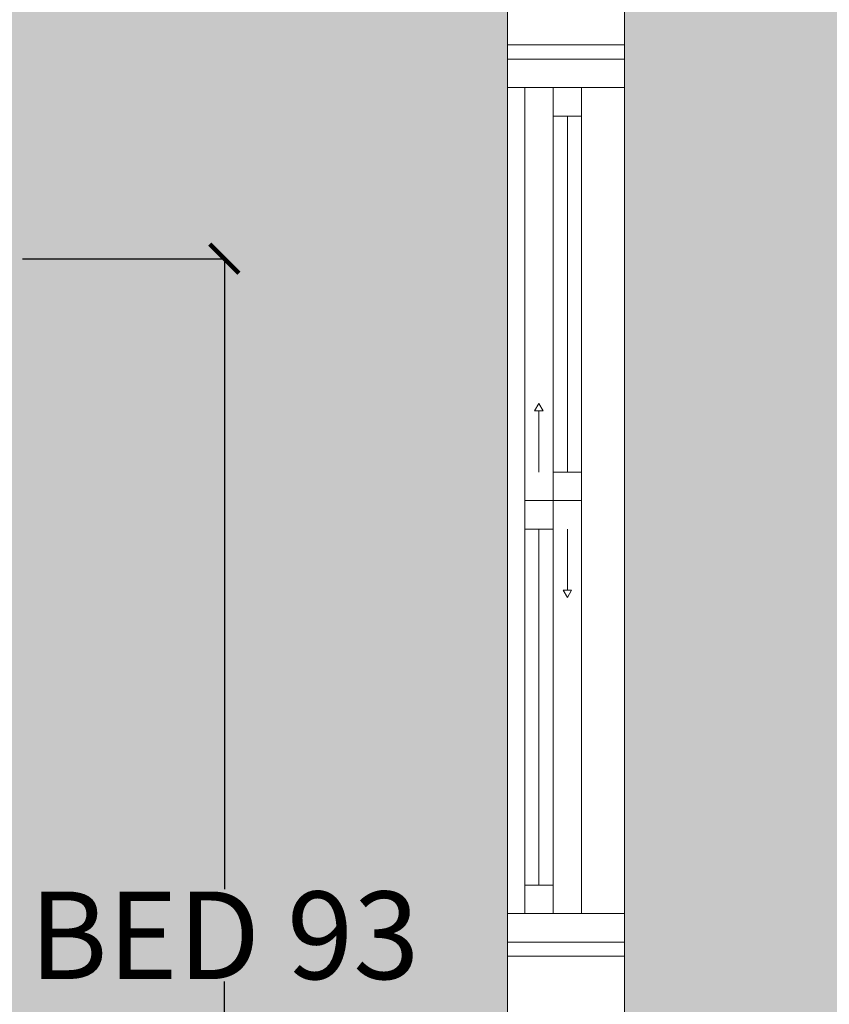
# Model space of a CAD drawing. Units: inches. Extents: x 1704 to 6393, y -157 to 1172.
# Tile 36 of 122: x 2564 to 2619, y 148 to 215. Entities that reach past the tile are written whole.
import ezdxf

# ---------------------------------------------------------------- set-up
doc = ezdxf.new("R2010")
doc.units = ezdxf.units.IN
doc.header["$MEASUREMENT"] = 0
for name, color, linetype, lineweight in [('A-ANNO-DIMS', 7, 'Continuous', 13), ('L-PVMT-PATT', 8, 'Continuous', 13), ('WINDOWS', 2, 'Continuous', 18)]:
    doc.layers.add(name, color=color, linetype=linetype, lineweight=lineweight)
doc.layers.add('A-FLOR-PATT', color=7, linetype='Continuous', lineweight=13, true_color=0xf2f2f2)
doc.layers.add('L-HRDS-PATT', color=9, linetype='Continuous', lineweight=13, true_color=0xc5c1ba)
doc.styles.get("Standard").update_dxf_attribs({"font": 'arial.ttf'})
doc.dimstyles.get("Standard").update_dxf_attribs({"dimtxt": 6, "dimasz": 2, "dimexe": 0.18, "dimexo": 0.0625, "dimgap": 0.09, "dimtad": 0, "dimtih": 1, "dimtoh": 1, "dimdec": 1, "dimzin": 0, "dimdsep": 46, "dimlunit": 3, "dimtxsty": 'Standard', "dimblk": 'ARCHTICK', "dimcen": 0.09, "dimadec": 0, "dimazin": 0, "dimtfac": 1, "dimtdec": 1, "dimtofl": 0, "dimtmove": 0, "dimatfit": 3, "dimfxl": 1, "dimtolj": 1, "dimtzin": 0, "dimarcsym": 0})

# ---------------------------------------------------------------- blocks, each defined once
blk = doc.blocks.new('WIN-SLIDER-72')
for p, q in [((-0.0004259439410816, 71.9999735309789), (-0.0004259439410816, -2.6469021094e-05)), ((7.999574056058918, 66.25124978916168), (7.999574056058918, 71.9999735309789)), ((-0.0004259439410816, 67.22709741074826), (7.999574056058918, 67.22709741074826)), ((1.168640707413942, 35.99997353097891), (1.168640707413942, 64.29955454714539)), ((7.999574056058918, 7.700392514812421), (7.999574056058918, 64.29955454714539)), ((3.120335949861328, 37.95166877356272), (3.120335949861328, 62.34785930456158)), ((4.09618357115869, 37.95166877356272), (4.09618357115869, 62.34785930456158)), ((5.072031192385111, 37.95166877356272), (5.072031192385111, 62.34785930456158)), ((2.144488328640363, 37.95166877356272), (2.144488328640363, 42.14359235372424)), ((5.072031192385111, 35.99997353097891), (5.072031192385111, 7.700392514812421)), ((1.168640707413942, 9.652087757418059), (1.168640707413942, 34.0482782883951)), ((2.144488328640363, 9.652087757418059), (2.144488328640363, 34.0482782883951)), ((3.120335949861328, 9.652087757418059), (3.120335949861328, 34.0482782883951)), ((4.09618357115869, 34.0482782883951), (4.09618357115869, 29.85635470823357)), ((7.999574056058918, 5.748697272796135), (7.999574056058918, -2.6469021094e-05)), ((-0.0004259439410816, 4.772849651209554), (7.999574056058918, 4.772849651209554))]:
    blk.add_line(p, q)
for points in [[(7.999574056058918, 64.29955454714539), (7.999574056058918, 66.25124978916168), (-0.0004259439410816, 66.25124978916168), (-0.0004259439410816, 64.29955454714539)], [(5.072031192385111, 62.34785930456158), (5.072031192385111, 64.29955454714539), (3.120335949861328, 64.29955454714539), (3.120335949861328, 62.34785930456158)], [(2.144488328640363, 42.64905607955327), (1.852658710451578, 42.14359235372424), (2.436317946894632, 42.14359235372424)], [(5.072031192385111, 35.99997353097891), (5.072031192385111, 37.95166877356272), (3.120335949861328, 37.95166877356272), (3.120335949861328, 35.99997353097891)], [(3.120335949861328, 34.0482782883951), (3.120335949861328, 35.99997353097891), (1.168640707413942, 35.99997353097891), (1.168640707413942, 34.0482782883951)], [(4.09618357115869, 29.35089098240453), (3.804353952904421, 29.85635470823357), (4.388013189347475, 29.85635470823357)], [(3.120335949861328, 7.700392514812421), (3.120335949861328, 9.652087757418059), (1.168640707413942, 9.652087757418059), (1.168640707413942, 7.700392514812421)], [(7.999574056058918, 7.700392514812421), (7.999574056058918, 5.748697272796135), (-0.0004259439410816, 5.748697272796135), (-0.0004259439410816, 7.700392514812421)]]:
    blk.add_lwpolyline(points, close=True)
blk = doc.blocks.new('_ArchTick')
at = {"color": 0, "linetype": 'ByBlock', "const_width": 0.15}
blk.add_lwpolyline([(-0.5, -0.5), (0.5, 0.5)], dxfattribs=at)
blk = doc.blocks.new('*D64')
at = {"layer": 'A-ANNO-DIMS', "color": 0, "lineweight": -2, "transparency": 16777216}
for p, q in [((2564.088538543452, 198.7857588392528), (2578.114519968197, 198.7857588392528)), ((2577.934519968197, 198.7857588392528), (2577.934519968197, 155.5796384011561)), ((2577.934519968197, 106.0625493409584), (2577.934519968197, 149.2686697790551)), ((2564.088538543452, 106.0625493409584), (2578.114519968197, 106.0625493409584))]:
    blk.add_line(p, q, dxfattribs=at)
at = {"layer": 'Defpoints', "color": 0, "lineweight": -3, "transparency": 16777216}
for p in [(2564.026038543452, 198.7857588392528), (2564.026038543452, 106.0625493409584), (2577.934519968197, 106.0625493409584)]:
    blk.add_point(p, dxfattribs=at)
at = {"layer": 'A-ANNO-DIMS', "color": 0, "lineweight": -2, "transparency": 16777216, "xscale": 2, "yscale": 2, "zscale": 2}
for p, rotation in [((2577.934519968197, 198.7857588392528), 90), ((2577.934519968197, 106.0625493409584), 270)]:
    blk.add_blockref('_ArchTick', p, dxfattribs=dict(at, rotation=rotation))
at = {"layer": 'A-ANNO-DIMS', "color": 0, "transparency": 16777216, "insert": (2577.934519968196, 152.4241540901048), "char_height": 6, "attachment_point": 5}
blk.add_mtext('\\A1;BED 93', dxfattribs=at)
blk = doc.blocks.new('*D93')
at = {"layer": 'A-ANNO-DIMS', "color": 0, "lineweight": -2, "transparency": 16777216}
for p, q in [((2605.286074000001, 895.2129740000005), (1829.697551000002, 895.2129740000003)), ((1829.877551000002, 895.2129740000003), (1829.877551000002, 495.8664119263302)), ((1829.877551000002, 90.2129739999999), (1829.877551000002, 489.5595360736699)), ((2605.286074000001, 90.21297400000003), (1829.697551000002, 90.2129739999999))]:
    blk.add_line(p, q, dxfattribs=at)
at = {"layer": 'Defpoints', "color": 0, "lineweight": -3, "transparency": 16777216}
for p in [(2605.348574000001, 895.2129740000005), (1829.877551000002, 90.2129739999999), (2605.348574000001, 90.21297400000003)]:
    blk.add_point(p, dxfattribs=at)
at = {"layer": 'A-ANNO-DIMS', "color": 0, "lineweight": -2, "transparency": 16777216, "xscale": 2, "yscale": 2, "zscale": 2}
for p, rotation in [((1829.877551000002, 895.2129740000003), 90), ((1829.877551000002, 90.2129739999999), 270)]:
    blk.add_blockref('_ArchTick', p, dxfattribs=dict(at, rotation=rotation))
at = {"layer": 'A-ANNO-DIMS', "color": 0, "transparency": 16777216, "insert": (1829.877551000001, 492.7129739999994), "char_height": 6, "attachment_point": 5}
blk.add_mtext('\\A1;805', dxfattribs=at)

msp = doc.modelspace()

# ---------------------------------------------------------------- hatches: boundary and pattern name
at = {"layer": 'A-FLOR-PATT', "transparency": 33554528}
h = msp.add_hatch(color=256, dxfattribs=at)
h.dxf.hatch_style = 1
h.paths.add_polyline_path([(2325.348574056059, 863.2129735309796), (2325.348574056059, 887.2129735309796), (2263.348574056059, 887.2129735309796), (2167.348574056059, 887.2129735309794), (2081.348574056061, 887.2129735309792), (2081.348574056061, 719.2129735309785), (2277.348574056059, 719.2129735309787), (2277.348574056059, 711.2129735309788), (2277.348574056059, 372.212973530979), (2349.348574056059, 372.212973530979), (2381.348574056059, 372.2129735309789), (2381.348574056059, 364.2129735309789), (2353.348574056059, 364.2129735309789), (2353.348574056059, 270.2129735309788), (2381.348574056059, 270.2129735309788), (2381.348574056059, 266.2129735309788), (2357.348574056059, 266.2129735309788), (2357.348574056059, 98.21297353097884), (2381.348574056059, 98.21297353097897), (2385.181056550604, 98.21297353097884), (2386.482186711948, 98.21297353097884), (2424.21496140017, 98.21297353097884), (2425.516091561514, 98.21297353097884), (2429.348574056059, 98.21297353097897), (2597.348574056059, 98.21297353097884), (2597.348574056059, 146.2129735309788), (2597.348574056059, 218.2129735309788), (2597.348574056059, 266.2129735309788), (2423.348574056059, 266.2129735309788), (2423.348574056059, 270.2129735309788), (2473.348574056059, 270.2129735309788), (2473.348574056059, 294.2129735309789), (2477.348574056059, 294.2129735309789), (2477.348574056059, 270.2129735309788), (2547.348574056059, 270.2129735309788), (2547.348574056059, 364.2129735309788), (2477.348574056059, 364.2129735309788), (2477.348574056059, 318.2129735309788), (2473.348574056059, 318.2129735309787), (2473.348574056059, 364.2129735309789), (2423.348574056059, 364.2129735309788), (2423.348574056059, 372.2129735309788), (2469.348574056059, 372.2129735309788), (2469.348574056059, 459.2129735309789), (2469.348574056059, 538.2129735309788), (2350.348574056059, 538.2129735309788), (2350.348574056059, 565.7129735309788), (2358.348574056059, 565.7129735309788), (2358.348574056059, 545.2129735309788), (2420.348574056059, 545.2129735309788), (2420.348574056059, 610.2129735309788), (2358.348574056059, 610.2129735309788), (2358.348574056059, 589.7129735309788), (2350.348574056059, 589.7129735309788), (2350.348574056059, 615.2129735309788), (2425.348574056059, 615.2129735309788), (2425.348574056059, 607.2129735309788), (2425.348574056059, 546.2129735309788), (2469.348574056059, 546.2129735309788), (2514.34857405606, 546.212973530979), (2514.34857405606, 607.2129735309788), (2449.348574056059, 607.2129735309788), (2449.348574056059, 615.2129735309788), (2451.737974987759, 615.2129735309788), (2451.737974987759, 659.2129735309788), (2427.737974987759, 659.2129735309788), (2427.737974987759, 665.2129735309788), (2367.737974987758, 665.2129735309788), (2367.737974987758, 667.2129735309788), (2367.737974987758, 711.2129735309788), (2325.348574056059, 711.2129735309788), (2325.348574056059, 719.2129735309785), (2325.348574056059, 755.2129735309787), (2325.348574056059, 763.2129735309788)])
h.paths.add_polyline_path([(2233.85817000392, 822.532660166629, -0.1872470486944155), (2233.85817000392, 809.1396667958562), (2231.697030374885, 808.8044951349628, 0.0848927708004382), (2233.130501812631, 814.4858417746204), (2230.423974436808, 814.4858417746204, -0.1042581087707907), (2228.553363812687, 808.3129425443484), (2217.750790159711, 807.1555239386723, -0.2222222222222219), (2217.750790159711, 824.5168030238124), (2228.553363812687, 823.3593844181363, -0.1042581087707933), (2230.423974436808, 817.1864851878643), (2233.130501812631, 817.1864851878643, 0.08489277080044), (2231.697030374885, 822.8678318275219)], flags=16)
h.paths.add_polyline_path([(2213.621360876743, 833.1974425663823), (2213.621360876743, 798.4748843961024), (2156.047684459484, 798.4748843961034), (2156.047684459485, 833.1974425663813)], flags=16)
h.paths.add_polyline_path([(2203.931929661768, 848.0987249710489), (2205.089348267444, 837.2961513180724, -0.2222222222222264), (2187.728069182304, 837.2961513180724), (2188.88548778798, 848.0987249710485, -0.104258108770792), (2195.058387018252, 849.9693355951691), (2195.058387018252, 852.6758629709927, 0.084892770800438), (2189.377040378595, 851.2423915332469), (2189.712212039488, 853.4035311622828, -0.1872470486944166), (2203.105205410261, 853.4035311622828), (2203.440377071154, 851.2423915332469, 0.084892770800438), (2197.759030431496, 852.6758629709927), (2197.759030431496, 849.9693355951691, -0.1042581087707896)], flags=16)
h.paths.add_polyline_path([(2181.940976153924, 837.2961513180726, -0.2222222222222323), (2164.579697068783, 837.2961513180724), (2165.73711567446, 848.0987249710487, -0.1042581087707905), (2171.910014904732, 849.9693355951691), (2171.910014904732, 852.6758629709927, 0.0848927708004445), (2166.228668265074, 851.2423915332469), (2166.563839925967, 853.403531162283, -0.1872470486944096), (2179.95683329674, 853.4035311622828), (2180.292004957633, 851.2423915332465, 0.0848927708004458), (2174.610658317976, 852.6758629709927), (2174.610658317976, 849.9693355951691, -0.104258108770801), (2180.783557548248, 848.0987249710482)], flags=16)
h.paths.add_polyline_path([(2205.089348267444, 794.376175644412), (2203.931929661768, 783.5736019914364, -0.1042581087707934), (2197.759030431496, 781.7029913673155), (2197.759030431496, 778.9964639914921, 0.084892770800439), (2203.440377071154, 780.4299354292382), (2203.105205410261, 778.2687958002022, -0.1872470486944172), (2189.712212039488, 778.2687958002018), (2189.377040378595, 780.4299354292377, 0.0848927708004369), (2195.058387018252, 778.9964639914919), (2195.058387018252, 781.7029913673153, -0.1042581087707904), (2188.88548778798, 783.5736019914358), (2187.728069182304, 794.3761756444126, -0.2222222222222231)], flags=16)
h.paths.add_polyline_path([(2181.940976153924, 794.376175644412), (2180.783557548248, 783.5736019914364, -0.1042581087708008), (2174.610658317976, 781.7029913673153), (2174.610658317976, 778.9964639914921, 0.0848927708004458), (2180.292004957633, 780.4299354292382), (2179.95683329674, 778.268795800202, -0.1872470486944096), (2166.563839925967, 778.2687958002018), (2166.228668265074, 780.4299354292378, 0.0848927708004446), (2171.910014904732, 778.9964639914919), (2171.910014904732, 781.7029913673153, -0.1042581087707904), (2165.73711567446, 783.5736019914358), (2164.579697068783, 794.3761756444123, -0.2222222222222294)], flags=16)
h.paths.add_polyline_path([(2151.918255176517, 807.1555239386723), (2141.115681523541, 808.3129425443484, -0.1042581087707911), (2139.24507089942, 814.4858417746204), (2136.538543523597, 814.4858417746204, 0.08489277080044), (2137.972014961343, 808.8044951349626), (2135.810875332307, 809.1396667958562, -0.1872470486944109), (2135.810875332307, 822.5326601666285), (2137.972014961343, 822.8678318275221, 0.0848927708004416), (2136.538543523597, 817.1864851878643), (2139.24507089942, 817.1864851878643, -0.104258108770793), (2141.115681523541, 823.3593844181363), (2151.918255176517, 824.5168030238124, -0.2222222222222205)], flags=16)
h.paths.add_polyline_path([(2357.868011454448, 363.4102250290031), (2358.813881560335, 363.4102250290031, 0.7537604849588476)], flags=16)
h.paths.add_polyline_path([(2372.241054283868, 363.1167008961685), (2372.248110816919, 363.1167008961685), (2372.248110816919, 363.3425764997267), (2371.30224071103, 363.3425764997267), (2371.30224071103, 363.1392706554335, -1.360391292333951)], flags=16)
h.paths.add_polyline_path([(2371.309297244092, 272.7157694655011), (2371.30224071103, 272.7157694655011), (2371.30224071103, 272.4898938619428), (2372.248110816919, 272.4898938619428), (2372.248110816919, 272.6931997062759, -1.360391292393621)], flags=16)
h.paths.add_polyline_path([(2357.875067987504, 272.7157694655011), (2357.868011454452, 272.7157694655011), (2357.868011454452, 272.4898938619428), (2358.813881560341, 272.4898938619428), (2358.813881560341, 272.6931997062361, -1.360391292333948)], flags=16)
h.paths.add_polyline_path([(2353.768696905258, 363.0736921025416), (2376.347425366111, 363.0736921025416), (2376.347425366111, 272.7587782591281), (2353.768696905258, 272.7587782591281)], flags=16)
h.paths.add_polyline_path([(2354.772195947961, 362.0701930598379), (2375.343926323407, 362.0701930598379), (2375.343926323407, 273.7622773018316), (2354.772195947961, 273.7622773018318)], flags=0)
h.paths.add_polyline_path([(2357.868011454452, 363.3425764997267), (2358.813881560341, 363.3425764997266), (2358.813881560341, 363.1167008961684), (2357.868011454452, 363.1167008961684)], flags=16)
h.paths.add_polyline_path([(2359.287941640134, 359.1843485433627), (2359.287941640134, 360.0631949744305), (2370.828180631237, 360.0631949744362), (2370.828180631237, 359.1843485433769), (2374.332057422314, 359.1843485433812), (2374.332057422312, 358.4635369582513), (2372.835178716611, 358.4635369582524), (2372.835178716611, 357.5410357047662), (2374.332057422314, 357.5410357047678), (2374.332057422312, 356.8202241196381), (2372.835178716611, 356.820224119639), (2372.835178716611, 355.897722866153), (2374.332057422314, 355.8977228661546), (2374.332057422312, 355.1769112810248), (2372.835178716611, 355.1769112810259), (2372.835178716611, 354.2544100275397), (2374.332057422334, 354.2544100275415), (2374.332057422331, 353.5335984424117), (2372.835178716631, 353.5335984424126), (2372.835178716631, 352.6110971889265), (2374.332057422334, 352.6110971889282), (2374.332057422331, 351.8902856037984), (2372.835178716631, 351.8902856037993), (2372.835178716631, 350.9677843503132), (2374.332057422334, 350.967784350315), (2374.332057422331, 350.2469727651852), (2372.835178716631, 350.2469727651861), (2372.835178716631, 349.3244715117), (2374.332057422334, 349.3244715117017), (2374.332057422331, 348.603659926572), (2372.835178716631, 348.6036599265729), (2372.835178716631, 347.6811586730868), (2374.332057422334, 347.6811586730886), (2374.332057422331, 346.9603470879587), (2372.835178716631, 346.9603470879598), (2372.835178716631, 346.0378458344735), (2374.332057422334, 346.0378458344753), (2374.332057422331, 345.3170342493456), (2372.835178716631, 345.3170342493465), (2372.835178716631, 344.3945329958605), (2374.332057422334, 344.3945329958621), (2374.332057422331, 343.6737214107324), (2372.835178716631, 343.6737214107334), (2372.835178716631, 342.751220157247), (2374.332057422334, 342.7512201572489), (2374.332057422331, 342.0304085721191), (2372.835178716631, 342.03040857212), (2372.835178716631, 341.1079073186338), (2374.332057422334, 341.1079073186356), (2374.332057422331, 340.3870957335057), (2372.835178716631, 340.3870957335066), (2372.835178716631, 339.4645944800207), (2374.332057422334, 339.4645944800223), (2374.332057422331, 338.7437828948924), (2372.835178716648, 338.7437828948933), (2372.835178716648, 337.8212816414076), (2374.332057422334, 337.8212816414093), (2374.332057422331, 337.1004700562794), (2372.835178716648, 337.1004700562803), (2372.835178716648, 336.1779688027942), (2374.332057422334, 336.1779688027961), (2374.332057422331, 335.4571572176662), (2372.835178716648, 335.4571572176673), (2372.835178716648, 334.5346559641809), (2374.332057422334, 334.5346559641828), (2374.332057422331, 333.8138443790529), (2372.835178716648, 333.8138443790539), (2372.835178716648, 332.8913431255679), (2374.332057422334, 332.8913431255696), (2374.332057422331, 332.1705315404397), (2372.835178716648, 332.1705315404406), (2372.835178716648, 331.2480302869545), (2374.332057422334, 331.2480302869563), (2374.332057422331, 330.5272187018265), (2372.835178716648, 330.5272187018273), (2372.835178716648, 329.6047174483413), (2374.332057422334, 329.6047174483431), (2374.332057422331, 328.8839058632133), (2372.835178716648, 328.8839058632143), (2372.835178716648, 327.9614046097282), (2374.332057422334, 327.9614046097298), (2374.332057422331, 327.2405930246), (2372.835178716648, 327.2405930246009), (2372.835178716648, 326.3180917711149), (2374.332057422334, 326.3180917711167), (2374.332057422331, 325.5972801859869), (2372.835178716648, 325.5972801859877), (2372.835178716648, 324.6747789325016), (2374.332057422334, 324.6747789325034), (2374.332057422331, 323.9539673473736), (2372.835178716648, 323.9539673473746), (2372.835178716648, 323.0314660938884), (2374.332057422334, 323.0314660938901), (2374.332057422331, 322.3106545087603), (2372.835178716648, 322.3106545087613), (2372.835178716648, 321.3881532552753), (2374.332057422334, 321.388153255277), (2374.332057422331, 320.6673416701471), (2372.835178716648, 320.6673416701481), (2372.835178716648, 319.7448404166621), (2374.332057422334, 319.7448404166638), (2374.332057422331, 319.0240288315339), (2372.835178716648, 319.0240288315348), (2372.835178716648, 318.1015275780487), (2374.332057422334, 318.1015275780504), (2374.332057422331, 317.3807159929205), (2372.835178716648, 317.3807159929214), (2372.835178716648, 316.4582147394357), (2374.332057422334, 316.4582147394373), (2374.332057422331, 315.7374031543073), (2372.835178716648, 315.7374031543084), (2372.835178716648, 314.8149019008223), (2374.332057422334, 314.8149019008241), (2374.332057422331, 314.0940903156943), (2372.835178716648, 314.0940903156952), (2372.835178716648, 313.171589062209), (2374.332057422334, 313.1715890622108), (2374.332057422331, 312.450777477081), (2372.835178716648, 312.4507774770819), (2372.835178716648, 311.5282762235959), (2374.332057422334, 311.5282762235977), (2374.332057422331, 310.8074646384678), (2372.835178716648, 310.8074646384687), (2372.835178716648, 309.8849633849827), (2374.332057422334, 309.8849633849844), (2374.332057422331, 309.1641517998546), (2372.835178716648, 309.1641517998555), (2372.835178716648, 308.2416505463693), (2374.332057422334, 308.2416505463712), (2374.332057422331, 307.5208389612412), (2372.835178716648, 307.5208389612421), (2372.835178716648, 306.5983377077562), (2374.332057422334, 306.598337707758), (2374.332057422331, 305.8775261226281), (2372.835178716648, 305.8775261226289), (2372.835178716648, 304.955024869143), (2374.332057422334, 304.9550248691447), (2374.332057422331, 304.2342132840149), (2372.835178716648, 304.2342132840158), (2372.835178716648, 303.3117120305298), (2374.332057422334, 303.3117120305316), (2374.332057422331, 302.5909004454018), (2372.835178716648, 302.5909004454027), (2372.835178716648, 301.6683991919165), (2374.332057422334, 301.6683991919183), (2374.332057422331, 300.9475876067885), (2372.835178716648, 300.9475876067894), (2372.835178716648, 300.0250863533033), (2374.332057422334, 300.025086353305), (2374.332057422331, 299.3042747681752), (2372.835178716648, 299.3042747681761), (2372.835178716648, 298.3817735146902), (2374.332057422334, 298.3817735146919), (2374.332057422331, 297.6609619295621), (2372.835178716648, 297.6609619295629), (2372.835178716648, 296.7384606760769), (2374.332057422334, 296.7384606760786), (2374.332057422331, 296.0176490909488), (2372.835178716648, 296.0176490909498), (2372.835178716648, 295.0951478374636), (2374.332057422334, 295.0951478374653), (2374.332057422331, 294.3743362523355), (2372.835178716648, 294.3743362523364), (2372.835178716648, 293.4518349988504), (2374.332057422334, 293.4518349988522), (2374.332057422331, 292.7310234137224), (2372.835178716648, 292.7310234137233), (2372.835178716648, 291.8085221602371), (2374.332057422334, 291.8085221602389), (2374.332057422331, 291.0877105751091), (2372.835178716648, 291.08771057511), (2372.835178716648, 290.165209321624), (2374.332057422334, 290.1652093216256), (2374.332057422331, 289.4443977364957), (2372.835178716648, 289.4443977364966), (2372.835178716648, 288.5218964830108), (2374.332057422334, 288.5218964830125), (2374.332057422331, 287.8010848978827), (2372.835178716648, 287.8010848978836), (2372.835178716648, 286.8785836443975), (2374.332057422334, 286.8785836443993), (2374.332057422331, 286.1577720592695), (2372.835178716648, 286.1577720592703), (2372.835178716648, 285.2352708057842), (2374.332057422334, 285.2352708057861), (2374.332057422331, 284.5144592206562), (2372.835178716648, 284.514459220657), (2372.835178716648, 283.5919579671712), (2374.332057422334, 283.5919579671728), (2374.332057422331, 282.871146382043), (2372.835178716648, 282.8711463820439), (2372.835178716648, 281.9486451285579), (2374.332057422334, 281.9486451285596), (2374.332057422331, 281.2278335434298), (2372.835178716648, 281.2278335434307), (2372.835178716648, 280.3053322899446), (2374.332057422334, 280.3053322899464), (2374.332057422331, 279.5845207048164), (2372.835178716648, 279.5845207048174), (2372.835178716648, 278.6620194513314), (2374.332057422334, 278.6620194513331), (2374.332057422331, 277.9412078662033), (2372.835178716648, 277.9412078662043), (2372.835178716648, 277.0187066127184), (2374.332057422334, 277.0187066127201), (2374.332057422331, 276.29789502759), (2370.828180631244, 276.2978950275922), (2370.828180631244, 275.7692753872335), (2359.287941640128, 275.7692753872392), (2359.287941640128, 276.2978950275993), (2355.784064849037, 276.2978950276015), (2355.784064849037, 277.0187066126971), (2357.280943554723, 277.0187066126989), (2357.280943554723, 277.9412078662137), (2355.784064849037, 277.9412078662145), (2355.784064849037, 278.6620194513103), (2357.280943554723, 278.6620194513122), (2357.280943554723, 279.5845207048271), (2355.784064849037, 279.584520704828), (2355.784064849037, 280.3053322899236), (2357.280943554723, 280.3053322899253), (2357.280943554723, 281.2278335434403), (2355.784064849037, 281.2278335434412), (2355.784064849037, 281.9486451285369), (2357.280943554723, 281.9486451285387), (2357.280943554723, 282.8711463820535), (2355.784064849037, 282.8711463820543), (2355.784064849037, 283.5919579671501), (2357.280943554723, 283.591957967152), (2357.280943554723, 284.5144592206668), (2355.784064849037, 284.5144592206676), (2355.784064849037, 285.2352708057632), (2357.280943554723, 285.2352708057651), (2357.280943554723, 286.1577720592801), (2355.784064849037, 286.1577720592809), (2355.784064849037, 286.8785836443766), (2357.280943554723, 286.8785836443784), (2357.280943554723, 287.8010848978931), (2355.784064849037, 287.8010848978941), (2355.784064849037, 288.5218964829895), (2357.280943554723, 288.5218964829913), (2357.280943554723, 289.4443977365064), (2355.784064849037, 289.4443977365072), (2355.784064849037, 290.1652093216029), (2357.280943554723, 290.1652093216047), (2357.280943554723, 291.0877105751197), (2355.784064849037, 291.0877105751206), (2355.784064849037, 291.8085221602161), (2357.280943554723, 291.8085221602179), (2357.280943554723, 292.7310234137328), (2355.784064849037, 292.7310234137337), (2355.784064849037, 293.4518349988293), (2357.280943554723, 293.451834998831), (2357.280943554723, 294.3743362523461), (2355.784064849037, 294.3743362523469), (2355.784064849037, 295.0951478374426), (2357.280943554723, 295.0951478374445), (2357.280943554723, 296.0176490909594), (2355.784064849037, 296.0176490909601), (2355.784064849037, 296.7384606760557), (2357.280943554723, 296.7384606760575), (2357.280943554723, 297.6609619295724), (2355.784064849037, 297.6609619295734), (2355.784064849037, 298.3817735146691), (2357.280943554723, 298.3817735146709), (2357.280943554723, 299.3042747681858), (2355.784064849037, 299.3042747681866), (2355.784064849037, 300.0250863532823), (2357.280943554723, 300.0250863532841), (2357.280943554723, 300.9475876067989), (2355.784064849037, 300.9475876067997), (2355.784064849037, 301.6683991918954), (2357.280943554723, 301.6683991918973), (2357.280943554723, 302.5909004454123), (2355.784064849037, 302.5909004454133), (2355.784064849037, 303.3117120305088), (2357.280943554723, 303.3117120305105), (2357.280943554723, 304.2342132840254), (2355.784064849037, 304.2342132840262), (2355.784064849037, 304.9550248691219), (2357.280943554723, 304.9550248691238), (2357.280943554723, 305.8775261226386), (2355.784064849037, 305.8775261226394), (2355.784064849037, 306.5983377077352), (2357.280943554723, 306.5983377077369), (2357.280943554723, 307.5208389612518), (2355.784064849037, 307.5208389612528), (2355.784064849037, 308.2416505463484), (2357.280943554723, 308.2416505463501), (2357.280943554723, 309.1641517998652), (2355.784064849037, 309.1641517998661), (2355.784064849037, 309.8849633849617), (2357.280943554723, 309.8849633849634), (2357.280943554723, 310.8074646384782), (2355.784064849037, 310.8074646384791), (2355.784064849037, 311.5282762235748), (2357.280943554723, 311.5282762235767), (2357.280943554723, 312.4507774770916), (2355.784064849037, 312.4507774770925), (2355.784064849037, 313.171589062188), (2357.280943554723, 313.1715890621898), (2357.280943554723, 314.0940903157049), (2355.784064849037, 314.0940903157058), (2355.784064849037, 314.8149019008013), (2357.280943554723, 314.8149019008032), (2357.280943554723, 315.7374031543179), (2355.784064849037, 315.7374031543187), (2355.784064849037, 316.4582147394146), (2357.280943554723, 316.4582147394165), (2357.280943554723, 317.3807159929311), (2355.784064849037, 317.3807159929321), (2355.784064849037, 318.1015275780277), (2357.280943554723, 318.1015275780295), (2357.280943554723, 319.0240288315445), (2355.784064849037, 319.0240288315454), (2355.784064849037, 319.744840416641), (2357.280943554723, 319.7448404166428), (2357.280943554723, 320.6673416701576), (2355.784064849037, 320.6673416701585), (2355.784064849037, 321.3881532552541), (2357.280943554723, 321.388153255256), (2357.280943554723, 322.3106545087708), (2355.784064849037, 322.3106545087718), (2355.784064849037, 323.0314660938674), (2357.280943554723, 323.0314660938692), (2357.280943554723, 323.9539673473843), (2355.784064849037, 323.9539673473851), (2355.784064849037, 324.6747789324806), (2357.280943554723, 324.6747789324824), (2357.280943554723, 325.5972801859974), (2355.784064849037, 325.5972801859983), (2355.784064849037, 326.3180917710939), (2357.280943554723, 326.3180917710958), (2357.280943554723, 327.2405930246105), (2355.784064849037, 327.2405930246113), (2355.784064849037, 327.9614046097071), (2357.280943554723, 327.961404609709), (2357.280943554723, 328.8839058632238), (2355.784064849037, 328.8839058632245), (2355.784064849037, 329.6047174483202), (2357.280943554723, 329.604717448322), (2357.280943554723, 330.527218701837), (2355.784064849037, 330.5272187018379), (2355.784064849037, 331.2480302869335), (2357.280943554723, 331.2480302869353), (2357.280943554723, 332.1705315404502), (2355.784064849037, 332.170531540451), (2355.784064849037, 332.8913431255468), (2357.280943554723, 332.8913431255486), (2357.280943554723, 333.8138443790634), (2355.784064849037, 333.8138443790642), (2355.784064849037, 334.5346559641599), (2357.280943554723, 334.5346559641618), (2357.280943554723, 335.4571572176767), (2355.784064849037, 335.4571572176776), (2355.784064849037, 336.1779688027732), (2357.280943554723, 336.177968802775), (2357.280943554723, 337.1004700562898), (2355.784064849037, 337.1004700562908), (2355.784064849037, 337.8212816413864), (2357.280943554723, 337.8212816413883), (2357.280943554723, 338.7437828949031), (2355.784064849037, 338.743782894904), (2355.784064849037, 339.4645944799996), (2357.280943554706, 339.4645944800013), (2357.280943554706, 340.3870957335163), (2355.784064849037, 340.3870957335173), (2355.784064849037, 341.1079073186129), (2357.280943554706, 341.1079073186146), (2357.280943554706, 342.0304085721296), (2355.784064849037, 342.0304085721304), (2355.784064849037, 342.7512201572262), (2357.280943554706, 342.751220157228), (2357.280943554706, 343.6737214107429), (2355.784064849037, 343.6737214107437), (2355.784064849037, 344.3945329958394), (2357.280943554706, 344.3945329958412), (2357.280943554706, 345.317034249356), (2355.784064849037, 345.3170342493569), (2355.784064849037, 346.0378458344526), (2357.280943554706, 346.0378458344544), (2357.280943554706, 346.9603470879692), (2355.784064849037, 346.9603470879701), (2355.784064849037, 347.6811586730658), (2357.280943554706, 347.6811586730677), (2357.280943554706, 348.6036599265824), (2355.784064849037, 348.6036599265833), (2355.784064849037, 349.324471511679), (2357.280943554706, 349.3244715116809), (2357.280943554706, 350.2469727651956), (2355.784064849037, 350.2469727651966), (2355.784064849037, 350.9677843502922), (2357.280943554706, 350.9677843502939), (2357.280943554706, 351.8902856038089), (2355.784064849037, 351.8902856038098), (2355.784064849037, 352.6110971889055), (2357.280943554706, 352.6110971889072), (2357.280943554706, 353.5335984424222), (2355.784064849037, 353.533598442423), (2355.784064849037, 354.2544100275187), (2357.280943554686, 354.2544100275204), (2357.280943554686, 355.1769112810354), (2355.784064849017, 355.1769112810362), (2355.784064849017, 355.897722866132), (2357.280943554686, 355.8977228661338), (2357.280943554686, 356.8202241196486), (2355.784064849017, 356.8202241196495), (2355.784064849017, 357.5410357047453), (2357.280943554686, 357.5410357047471), (2357.280943554686, 358.4635369582618), (2355.784064849017, 358.4635369582626), (2355.784064849017, 359.1843485433584)], flags=0)
at = {"layer": 'L-HRDS-PATT', "transparency": 33554539}
h = msp.add_hatch(color=256, dxfattribs=at)
h.dxf.hatch_style = 1
h.paths.add_polyline_path([(2651.216564110692, 368.2129735309789), (2605.348574056059, 368.2129735309789), (2605.348574056059, 218.2129735309789), (2605.348574056059, 212.4642497891616), (2605.348574056059, 210.5125545471454), (2605.348574056059, 153.9133925148124), (2605.348574056059, 151.9616972727961), (2605.348574056059, 146.2129735309789), (2605.348574056059, 90.21297353097891), (2605.348574056059, 72.21297353097891), (2601.348574056059, 72.21297353097891), (2600.87998259587, 50.63430582669659), (2719.348574056059, 50.63430582669662), (2719.348574056059, 72.2129735309789), (2711.348574056059, 72.2129735309789), (2663.216564110693, 72.2129735309789), (2651.216564110692, 72.2129735309789)])
h.paths.add_polyline_path([(2711.348574056059, 48.63430582669661), (2600.87998259587, 48.63430582669661), (2576.879982595869, 48.63430582669661), (2576.879982595869, 17.65795537009174), (2711.348574056059, 17.65795537009174)])
h.paths.add_polyline_path([(2601.348574056059, 72.21297353097891), (2597.348574056059, 72.2129735309789), (2597.348574056059, 90.21297353097891), (2429.34857405606, 90.21297353097891), (2425.516091561515, 90.21297353098161), (2424.214961400171, 90.21297353098161), (2386.482186711949, 90.21297353098161), (2385.181056550604, 90.21297353098161), (2381.34857405606, 90.21297353098161), (2357.348574056059, 90.21297353097891), (2357.348574056059, 72.21297353097891), (2349.348574056059, 72.21297353097891), (2349.348574056059, 90.21297353097891), (2349.348574056059, 134.2129735309789), (2277.348574056059, 134.2129735309789), (2277.348574056059, 50.63430582669662), (2566.87998259587, 50.63430582669662), (2600.87998259587, 50.63430582669662)])
h.paths.add_polyline_path([(2349.348574056059, 146.2129735309789), (2277.348574056059, 146.2129735309789), (2277.348574056059, 134.2129735309789), (2349.348574056059, 134.2129735309789)])
h.paths.add_polyline_path([(2349.348574056059, 158.2129735309789), (2277.348574056059, 158.2129735309789), (2277.348574056059, 146.2129735309789), (2349.348574056059, 146.2129735309789)])
h.paths.add_polyline_path([(2349.348574056059, 170.2129735309789), (2277.348574056059, 170.2129735309789), (2277.348574056059, 158.2129735309789), (2349.348574056059, 158.2129735309789)])
h.paths.add_polyline_path([(2349.348574056059, 194.212973530979), (2337.34857405606, 194.212973530979), (2337.34857405606, 202.212973530979), (2349.348574056059, 202.212973530979), (2349.348574056059, 364.212973530979), (2277.348574056059, 364.2129735309788), (2277.348574056059, 202.212973530979), (2289.348574056059, 202.212973530979), (2289.348574056059, 194.212973530979), (2277.348574056059, 194.2129735309789), (2277.348574056059, 170.2129735309789), (2349.348574056059, 170.2129735309789)])
at = {"layer": 'L-PVMT-PATT', "transparency": 33554643}
h = msp.add_hatch(dxfattribs=at)
h.set_pattern_fill('GRAVEL', color=256, scale=2.399999999999999)
h.set_pattern_definition([(228.012787504, (1.727999999999999, 2.399999999999999), (-19.20000000000015, -21.60000000000001), [0.3228864, -31.96581131297687]), (184.969740728, (1.512, 2.16), (28.79999999999994, 2.400000000000084), [0.5540832, -54.85421942695199]), (132.510447078, (0.9599999999999999, 2.112), (24.00000000000028, -26.39999999999968), [0.3906912, -38.67847823063928]), (267.273689006, (0.024, 1.512), (2.400000000000058, 48.00000000000004), [0.5045711999999999, -49.95253929990959]), (292.833654178, (0, 1.008), (-11.99999999999997, 28.80000000000007), [0.494772, -48.98249550741191]), (357.273689006, (0.192, 0.552), (-48.00000000000004, 2.400000000000061), [0.5045711999999999, -49.95253929990959]), (37.6942404667, (0.696, 0.5280000000000001), (-31.2, -23.99999999999994), [0.6672696, -66.0596365173984]), (72.2553283749, (1.223999999999999, 0.9359999999999999), (16.80000000000006, 52.80000000000001), [0.6299712, -62.36717159235214]), (121.429565615, (1.415999999999999, 1.536), (-19.20000000000004, 31.19999999999997), [0.50628, -50.12177546334959]), (175.236358309, (1.151999999999999, 1.967999999999999), (26.39999999999996, -2.40000000000009), [0.5779968000000001, -28.32183018910152]), (222.397437798, (0.576, 2.016), (-28.79999999999991, -26.39999999999993), [0.7474752000000001, -74.00010001150775]), (138.814074834, (2.399999999999999, 1.487999999999999), (-16.80000000000008, 14.4), [0.2551223999999999, -25.25722755056328]), (171.46923439, (2.208, 1.655999999999999), (31.2, -4.799999999999988), [0.4853688, -48.0516273987768]), (225, (1.727999999999999, 1.727999999999999), (-3e-16, -2.399999999999839), [0.3394104, -3.054702149695439]), (203.198590514, (1.56, 2.016), (11.99999999999997, 4.79999999999994), [0.1827792, -18.09507625407336]), (291.801409486, (1.391999999999999, 1.943999999999999), (-2.399999999999241, 7.200000000000246), [0.2584872, -12.6659083371228]), (30.96375653209999, (1.487999999999999, 1.703999999999999), (7.200000000000127, 4.79999999999995), [0.4198296, -13.57445494762872]), (161.565051177, (1.847999999999999, 1.919999999999999), (4.800000000000027, -2.399999999999943), [0.3035784, -7.285887984404157]), (16.389540334, (0, 1.943999999999999), (23.99999999999992, 7.200000000000104), [0.42528, -42.10282835200656]), (70.3461759419, (0.408, 2.064), (-9.600000000002929, -26.40000000000815), [0.3567863999999999, -35.3217785935656]), (293.198590514, (1.847999999999999, 2.399999999999999), (-4.799999999999928, 11.99999999999998), [0.365556, -17.91229945407336]), (343.610459666, (1.991999999999999, 2.064), (-23.99999999999992, 7.200000000000104), [0.42528, -42.10282835200558]), (339.44395478, (0, 0.456), (-12.00000000000009, 4.800000000000058), [0.4101119999999999, -20.09549698876199]), (294.775140569, (0.384, 0.312), (-12.00000000000001, 26.40000000000001), [0.3436272, -34.0191433518624]), (66.8014094864, (1.871999999999999, 0), (4.799999999999954, 11.99999999999993), [0.365556, -17.91229945407336]), (17.3540246363, (2.016, 0.336), (-31.19999999999994, -9.59999999999991), [0.4023144000000001, -39.829016674176]), (69.4439547804, (0.696, 0), (-4.800000000000016, -11.99999999999989), [0.2050559999999999, -20.300552988762]), (101.309932474, (1.727999999999999, 0), (-2.399999999999912, 9.60000000000003), [0.122376, -12.11527083262272]), (165.963756532, (1.703999999999999, 0.12), (7.1999999999999, -2.400000000000003), [0.4947720000000001, -9.40068150148248]), (186.009005957, (1.223999999999999, 0.24), (24.00000000000011, 2.399999999999959), [0.45852, -45.39341561890272]), (303.690067526, (1.487999999999999, 1.487999999999999), (-2.399999999999969, 4.799999999999966), [0.3461327999999999, -8.307190261113599]), (353.157226587, (1.679999999999999, 1.199999999999999), (40.80000000000003, -4.800000000000126), [0.6043056, -59.82615029766792]), (60.9453959009, (2.279999999999999, 1.127999999999999), (-9.599999999999941, -16.79999999999994), [0.2470944, -24.4624179383688]), (90, (2.399999999999999, 1.344), (-2.399999999999999, 2.399999999999999), [0.144, -2.255999999999999]), (120.256437164, (1.175999999999999, 0.312), (9.60000000000002, -16.80000000000002), [0.3334176, -33.00844797467952]), (48.01278750419999, (1.008, 0.6), (19.2, 21.59999999999994), [0.6457728, -31.64292491297687]), (0, (1.439999999999999, 1.08), (2.399999999999999, 2.399999999999999), [0.6240000000000001, -1.775999999999999]), (325.304846469, (2.064, 1.08), (24.00000000000033, -16.79999999999958), [0.3794735999999999, -37.56785832202079]), (254.0546040990001, (2.375999999999999, 0.864), (-2.40000000000009, -9.60000000000001), [0.3494448, -17.1228189342732]), (207.645975364, (2.279999999999999, 0.5280000000000001), (-45.59999999999988, -24.00000000000011), [0.5689560000000001, -56.32673803742255]), (175.42607874, (1.775999999999999, 0.264), (-31.19999999999989, 2.400000000000003), [0.6019176, -59.58977617912535])])
h.paths.add_polyline_path([(2719.348574056059, 368.2129735309789), (2711.348574056059, 368.2129735309789), (2711.348574056059, 318.4809302499189), (2663.216564110693, 318.4809302499189), (2663.216564110693, 368.2129735309789), (2651.216564110692, 368.2129735309789), (2651.216564110692, 72.2129735309789), (2663.216564110693, 72.2129735309789), (2663.216564110693, 137.2129735309789), (2711.348574056059, 137.2129735309789), (2711.348574056059, 72.21297353097893), (2663.216564110693, 72.2129735309789), (2651.216564110692, 72.2129735309789), (2651.216564110692, 368.2129735309789), (2605.348574056059, 368.2129735309788), (2605.348574056059, 218.2129735309789), (2605.348574056059, 212.4642497891616), (2605.348574056059, 210.5125545471454), (2605.348574056059, 153.9133925148124), (2605.348574056059, 151.9616972727961), (2605.348574056059, 146.2129735309789), (2605.348574056059, 90.21297353097891), (2605.348574056059, 72.2129735309789), (2601.348574056059, 72.2129735309789), (2600.87998259587, 50.63430582669662), (2277.348574056059, 50.63430582669659), (2277.348574056059, -3.787026469021128), (2719.348574056059, -3.787026469021185)])
h.paths.add_polyline_path([(2663.216564110693, 272.4809302499188), (2711.348574056059, 272.4809302499188), (2711.34857405606, 207.2129735309789), (2663.216564110693, 207.2129735309789)], flags=16)
h.paths.add_polyline_path([(2663.216564110693, 202.2129735309789), (2711.34857405606, 202.2129735309789), (2711.348574056059, 142.2129735309789), (2663.216564110693, 142.2129735309789)], flags=16)
h.paths.add_polyline_path([(2663.216564110693, 277.480930249925), (2663.216564110693, 313.4809302499188), (2711.348574056059, 313.4809302499188), (2711.348574056059, 277.4809302499189)], flags=16)

# ---------------------------------------------------------------- block references
at = {"layer": 'WINDOWS'}
msp.add_blockref('WIN-SLIDER-72', (2597.349, 146.213), dxfattribs=at)

# ---------------------------------------------------------------- dimensions: what is measured, and where the dimension line sits
at = {"layer": 'A-ANNO-DIMS'}
dim = msp.add_linear_dim(base=(1829.877551000002, 90.2129739999999), p1=(2605.348574000001, 895.212974), p2=(2605.348574000001, 90.21297399999999), angle=90, dimstyle='Standard', override={"dimdec": 0, "dimlfac": 1, "dimrnd": 0, "dimzin": 0, "dimdsep": 46, "dimlunit": 2}, dxfattribs=at)
dim.commit()
dim.dimension.update_dxf_attribs({"geometry": '*D93', "text_midpoint": (1829.877551000001, 492.7129739999994)})
dim = msp.add_linear_dim(base=(2577.934519968197, 106.0625493409584), p1=(2564.026038543451, 198.7857588392527), p2=(2564.026038543451, 106.0625493409584), angle=270, text='BED <>', dimstyle='Standard', override={"dimdec": 0, "dimlfac": 1, "dimrnd": 0, "dimzin": 0, "dimdsep": 46, "dimlunit": 2}, dxfattribs=at)
dim.commit()
dim.dimension.update_dxf_attribs({"geometry": '*D64', "text_midpoint": (2577.934519968196, 152.4241540901048)})

doc.saveas('drawing.dxf')
